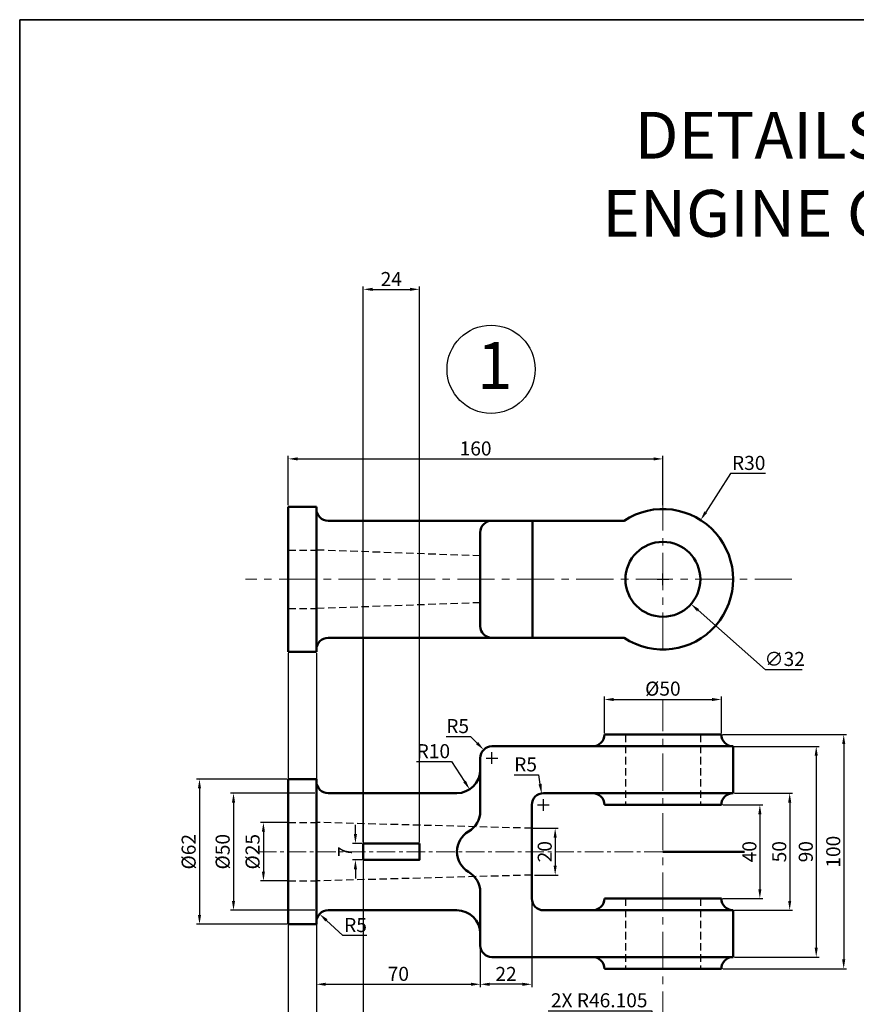
# Model space of a CAD drawing. Units: millimetres. Extents: x 208 to 901, y -26 to 704.
# Tile 2 of 3: x 208 to 566, y 283 to 704. Entities that reach past the tile are written whole.
import ezdxf

# ---------------------------------------------------------------- set-up
doc = ezdxf.new("R2010")
doc.units = ezdxf.units.MM
doc.header["$LTSCALE"] = 0.5
doc.linetypes.add('CENTER', pattern=[50.8, 31.75, -6.35, 6.35, -6.35])
doc.linetypes.add('DASHED', pattern=[19.05, 12.7, -6.35])
for name, color, linetype, lineweight in [('M-CNTR', 1, 'CENTER', 18), ('M-DIMS', 2, 'Continuous', 25), ('M-HIDN', 6, 'DASHED', 25), ('M-OUTL', 7, 'Continuous', 50), ('M-TEXT', 3, 'Continuous', 25), ('M-TTLB', 7, 'Continuous', 35)]:
    doc.layers.add(name, color=color, linetype=linetype, lineweight=lineweight)
doc.styles.get("Standard").update_dxf_attribs({"font": 'arial.ttf'})
doc.dimstyles.new('ISO-25', dxfattribs={"dimtxt": 6, "dimasz": 4, "dimexe": 1.25, "dimexo": 0.625, "dimtad": 1, "dimtoh": 1, "dimdec": 0, "dimtxsty": 'Standard', "dimcen": 2.5, "dimadec": 0, "dimazin": 0, "dimtfac": 1, "dimtdec": 0, "dimtofl": 0, "dimtmove": 0, "dimatfit": 3, "dimfxl": 1, "dimarcsym": 0})

# ---------------------------------------------------------------- blocks, each defined once
blk = doc.blocks.new('*D1')
at = {"layer": 'Defpoints', "color": 0, "ltscale": 0.5, "transparency": 16777216}
for p in [(483.01, 516.18), (323.01, 495.77), (483.01, 495.77)]:
    blk.add_point(p, dxfattribs=at)
at = {"layer": 'M-DIMS', "color": 0, "lineweight": -2, "ltscale": 0.5, "transparency": 16777216}
for p, q in [((323.01, 496.4), (323.01, 517.43)), ((483.01, 496.4), (483.01, 517.43)), ((327.01, 516.18), (479.01, 516.18))]:
    blk.add_line(p, q, dxfattribs=at)
at = {"layer": 'M-DIMS', "color": 0, "ltscale": 0.5, "transparency": 16777216}
for points in [[(327.01, 516.84), (327.01, 515.51), (323.01, 516.18)], [(479.01, 516.84), (479.01, 515.51), (483.01, 516.18)]]:
    blk.add_solid(points, dxfattribs=at)
at = {"layer": 'M-DIMS', "color": 0, "ltscale": 0.5, "transparency": 16777216, "insert": (403.01, 519.86), "char_height": 6, "attachment_point": 5}
blk.add_mtext('160', dxfattribs=at)
blk = doc.blocks.new('*D2')
at = {"layer": 'Defpoints', "color": 0, "ltscale": 0.5, "transparency": 16777216}
for p in [(471.01, 475.35), (495.02, 454.19)]:
    blk.add_point(p, dxfattribs=at)
at = {"layer": 'M-DIMS', "color": 0, "lineweight": -2, "ltscale": 0.5, "transparency": 16777216}
for p, q in [((483.01, 462.27), (483.01, 467.27)), ((480.51, 464.77), (485.51, 464.77)), ((526.89, 426.11), (498.02, 451.55)), ((542.57, 426.11), (526.89, 426.11))]:
    blk.add_line(p, q, dxfattribs=at)
at = {"layer": 'M-DIMS', "color": 0, "ltscale": 0.5, "transparency": 16777216}
blk.add_solid([(498.46, 452.05), (497.58, 451.05), (495.02, 454.19)], dxfattribs=at)
at = {"layer": 'M-DIMS', "color": 0, "ltscale": 0.5, "transparency": 16777216, "insert": (535.04, 429.96), "char_height": 6, "attachment_point": 5}
blk.add_mtext('∅32', dxfattribs=at)
blk = doc.blocks.new('*D3')
at = {"layer": 'Defpoints', "color": 0, "ltscale": 0.5, "transparency": 16777216}
for p in [(499.16, 490.06), (483.01, 464.77)]:
    blk.add_point(p, dxfattribs=at)
at = {"layer": 'M-DIMS', "color": 0, "lineweight": -2, "ltscale": 0.5, "transparency": 16777216}
for p, q in [((511.88, 509.99), (501.31, 493.43)), ((526.82, 509.99), (511.88, 509.99)), ((483.01, 462.27), (483.01, 467.27)), ((480.51, 464.77), (485.51, 464.77))]:
    blk.add_line(p, q, dxfattribs=at)
at = {"layer": 'M-DIMS', "color": 0, "ltscale": 0.5, "transparency": 16777216}
blk.add_solid([(500.75, 493.79), (501.87, 493.07), (499.16, 490.06)], dxfattribs=at)
at = {"layer": 'M-DIMS', "color": 0, "ltscale": 0.5, "transparency": 16777216, "insert": (519.67, 513.68), "char_height": 6, "attachment_point": 5}
blk.add_mtext('R30', dxfattribs=at)
blk = doc.blocks.new('*D4')
at = {"layer": 'Defpoints', "color": 0, "ltscale": 0.5, "transparency": 16777216}
for p in [(355.01, 351.93), (351.68, 344.93), (355.01, 344.93)]:
    blk.add_point(p, dxfattribs=at)
at = {"layer": 'M-DIMS', "color": 0, "lineweight": -2, "ltscale": 0.5, "transparency": 16777216}
for p, q in [((351.68, 355.93), (351.68, 359.93)), ((354.39, 351.93), (350.43, 351.93)), ((354.39, 344.93), (350.43, 344.93)), ((351.68, 340.93), (351.68, 336.93))]:
    blk.add_line(p, q, dxfattribs=at)
at = {"layer": 'M-DIMS', "color": 0, "ltscale": 0.5, "transparency": 16777216}
for points in [[(351.01, 355.93), (352.34, 355.93), (351.68, 351.93)], [(351.01, 340.93), (352.34, 340.93), (351.68, 344.93)]]:
    blk.add_solid(points, dxfattribs=at)
at = {"layer": 'M-DIMS', "color": 0, "ltscale": 0.5, "transparency": 16777216, "insert": (348.05, 348.43), "char_height": 6, "attachment_point": 5, "rotation": 90}
blk.add_mtext('7', dxfattribs=at)
blk = doc.blocks.new('*D5')
at = {"layer": 'Defpoints', "color": 0, "ltscale": 0.5, "transparency": 16777216}
for p in [(323.01, 360.93), (312.38, 335.93), (323.01, 335.93)]:
    blk.add_point(p, dxfattribs=at)
at = {"layer": 'M-DIMS', "color": 0, "lineweight": -2, "ltscale": 0.5, "transparency": 16777216}
for p, q in [((322.39, 360.93), (311.13, 360.93)), ((312.38, 356.93), (312.38, 339.93)), ((322.39, 335.93), (311.13, 335.93))]:
    blk.add_line(p, q, dxfattribs=at)
at = {"layer": 'M-DIMS', "color": 0, "ltscale": 0.5, "transparency": 16777216}
for points in [[(311.71, 356.93), (313.04, 356.93), (312.38, 360.93)], [(311.71, 339.93), (313.04, 339.93), (312.38, 335.93)]]:
    blk.add_solid(points, dxfattribs=at)
at = {"layer": 'M-DIMS', "color": 0, "ltscale": 0.5, "transparency": 16777216, "insert": (308.52, 348.43), "char_height": 6, "attachment_point": 5, "rotation": 90}
blk.add_mtext('%%C25', dxfattribs=at)
blk = doc.blocks.new('*D6')
at = {"layer": 'Defpoints', "color": 0, "ltscale": 0.5, "transparency": 16777216}
for p in [(335.01, 373.43), (299.6, 323.43), (335.01, 323.43)]:
    blk.add_point(p, dxfattribs=at)
at = {"layer": 'M-DIMS', "color": 0, "lineweight": -2, "ltscale": 0.5, "transparency": 16777216}
for p, q in [((334.39, 373.43), (298.35, 373.43)), ((299.6, 369.43), (299.6, 327.43)), ((334.39, 323.43), (298.35, 323.43))]:
    blk.add_line(p, q, dxfattribs=at)
at = {"layer": 'M-DIMS', "color": 0, "ltscale": 0.5, "transparency": 16777216}
for points in [[(298.93, 369.43), (300.27, 369.43), (299.6, 373.43)], [(298.93, 327.43), (300.27, 327.43), (299.6, 323.43)]]:
    blk.add_solid(points, dxfattribs=at)
at = {"layer": 'M-DIMS', "color": 0, "ltscale": 0.5, "transparency": 16777216, "insert": (295.74, 348.43), "char_height": 6, "attachment_point": 5, "rotation": 90}
blk.add_mtext('%%C50', dxfattribs=at)
blk = doc.blocks.new('*D7')
at = {"layer": 'Defpoints', "color": 0, "ltscale": 0.5, "transparency": 16777216}
for p in [(323.01, 379.43), (285.06, 317.43), (323.01, 317.43)]:
    blk.add_point(p, dxfattribs=at)
at = {"layer": 'M-DIMS', "color": 0, "lineweight": -2, "ltscale": 0.5, "transparency": 16777216}
for p, q in [((322.39, 379.43), (283.81, 379.43)), ((285.06, 375.43), (285.06, 321.43)), ((322.39, 317.43), (283.81, 317.43))]:
    blk.add_line(p, q, dxfattribs=at)
at = {"layer": 'M-DIMS', "color": 0, "ltscale": 0.5, "transparency": 16777216}
for points in [[(284.4, 375.43), (285.73, 375.43), (285.06, 379.43)], [(284.4, 321.43), (285.73, 321.43), (285.06, 317.43)]]:
    blk.add_solid(points, dxfattribs=at)
at = {"layer": 'M-DIMS', "color": 0, "ltscale": 0.5, "transparency": 16777216, "insert": (281.21, 348.43), "char_height": 6, "attachment_point": 5, "rotation": 90}
blk.add_mtext('%%C62', dxfattribs=at)
blk = doc.blocks.new('*D8')
at = {"layer": 'Defpoints', "color": 0, "ltscale": 0.5, "transparency": 16777216}
for p in [(335.01, 317.43), (405.01, 313.43), (405.01, 291.81)]:
    blk.add_point(p, dxfattribs=at)
at = {"layer": 'M-DIMS', "color": 0, "lineweight": -2, "ltscale": 0.5, "transparency": 16777216}
for p, q in [((335.01, 316.81), (335.01, 290.56)), ((405.01, 312.81), (405.01, 290.56)), ((339.01, 291.81), (401.01, 291.81))]:
    blk.add_line(p, q, dxfattribs=at)
at = {"layer": 'M-DIMS', "color": 0, "ltscale": 0.5, "transparency": 16777216}
for points in [[(339.01, 292.48), (339.01, 291.14), (335.01, 291.81)], [(401.01, 292.48), (401.01, 291.14), (405.01, 291.81)]]:
    blk.add_solid(points, dxfattribs=at)
at = {"layer": 'M-DIMS', "color": 0, "ltscale": 0.5, "transparency": 16777216, "insert": (370.01, 295.5), "char_height": 6, "attachment_point": 5}
blk.add_mtext('70', dxfattribs=at)
blk = doc.blocks.new('*D9')
at = {"layer": 'Defpoints', "color": 0, "ltscale": 0.5, "transparency": 16777216}
for p in [(427.01, 333.71), (405.01, 301.68), (405.01, 291.81)]:
    blk.add_point(p, dxfattribs=at)
at = {"layer": 'M-DIMS', "color": 0, "lineweight": -2, "ltscale": 0.5, "transparency": 16777216}
for p, q in [((427.01, 333.08), (427.01, 290.56)), ((405.01, 301.06), (405.01, 290.56)), ((423.01, 291.81), (409.01, 291.81))]:
    blk.add_line(p, q, dxfattribs=at)
at = {"layer": 'M-DIMS', "color": 0, "ltscale": 0.5, "transparency": 16777216}
for points in [[(409.01, 292.48), (409.01, 291.14), (405.01, 291.81)], [(423.01, 292.48), (423.01, 291.14), (427.01, 291.81)]]:
    blk.add_solid(points, dxfattribs=at)
at = {"layer": 'M-DIMS', "color": 0, "ltscale": 0.5, "transparency": 16777216, "insert": (416.01, 295.45), "char_height": 6, "attachment_point": 5}
blk.add_mtext('22', dxfattribs=at)
blk = doc.blocks.new('*D10')
at = {"layer": 'Defpoints', "color": 0, "ltscale": 0.5, "transparency": 16777216}
for p in [(427.01, 358.43), (427.56, 338.45), (437.01, 338.45)]:
    blk.add_point(p, dxfattribs=at)
at = {"layer": 'M-DIMS', "color": 0, "lineweight": -2, "ltscale": 0.5, "transparency": 16777216}
for p, q in [((427.64, 358.43), (438.26, 358.43)), ((437.01, 354.43), (437.01, 342.45)), ((428.18, 338.45), (438.26, 338.45))]:
    blk.add_line(p, q, dxfattribs=at)
at = {"layer": 'M-DIMS', "color": 0, "ltscale": 0.5, "transparency": 16777216}
for points in [[(436.34, 354.43), (437.67, 354.43), (437.01, 358.43)], [(436.34, 342.45), (437.67, 342.45), (437.01, 338.45)]]:
    blk.add_solid(points, dxfattribs=at)
at = {"layer": 'M-DIMS', "color": 0, "ltscale": 0.5, "transparency": 16777216, "insert": (433.32, 348.44), "char_height": 6, "attachment_point": 5, "rotation": 90}
blk.add_mtext('20', dxfattribs=at)
blk = doc.blocks.new('*D11')
at = {"layer": 'Defpoints', "color": 0, "ltscale": 0.5, "transparency": 16777216}
for p in [(508.01, 413.43), (458.01, 398.43), (508.01, 398.43)]:
    blk.add_point(p, dxfattribs=at)
at = {"layer": 'M-DIMS', "color": 0, "lineweight": -2, "ltscale": 0.5, "transparency": 16777216}
for p, q in [((458.01, 399.06), (458.01, 414.68)), ((462.01, 413.43), (504.01, 413.43)), ((508.01, 399.06), (508.01, 414.68))]:
    blk.add_line(p, q, dxfattribs=at)
at = {"layer": 'M-DIMS', "color": 0, "ltscale": 0.5, "transparency": 16777216}
for points in [[(462.01, 414.1), (462.01, 412.77), (458.01, 413.43)], [(504.01, 414.1), (504.01, 412.77), (508.01, 413.43)]]:
    blk.add_solid(points, dxfattribs=at)
at = {"layer": 'M-DIMS', "color": 0, "ltscale": 0.5, "transparency": 16777216, "insert": (483.01, 417.29), "char_height": 6, "attachment_point": 5}
blk.add_mtext('%%C50', dxfattribs=at)
blk = doc.blocks.new('*D12')
at = {"layer": 'Defpoints', "color": 0, "ltscale": 0.5, "transparency": 16777216}
for p in [(508.01, 368.43), (508.01, 328.43), (524.44, 328.43)]:
    blk.add_point(p, dxfattribs=at)
at = {"layer": 'M-DIMS', "color": 0, "lineweight": -2, "ltscale": 0.5, "transparency": 16777216}
for p, q in [((508.64, 368.43), (525.69, 368.43)), ((524.44, 364.43), (524.44, 332.43)), ((508.64, 328.43), (525.69, 328.43))]:
    blk.add_line(p, q, dxfattribs=at)
at = {"layer": 'M-DIMS', "color": 0, "ltscale": 0.5, "transparency": 16777216}
for points in [[(523.77, 364.43), (525.1, 364.43), (524.44, 368.43)], [(523.77, 332.43), (525.1, 332.43), (524.44, 328.43)]]:
    blk.add_solid(points, dxfattribs=at)
at = {"layer": 'M-DIMS', "color": 0, "ltscale": 0.5, "transparency": 16777216, "insert": (520.75, 348.43), "char_height": 6, "attachment_point": 5, "rotation": 90}
blk.add_mtext('40', dxfattribs=at)
blk = doc.blocks.new('*D13')
at = {"layer": 'Defpoints', "color": 0, "ltscale": 0.5, "transparency": 16777216}
for p in [(513.01, 373.43), (513.01, 323.43), (537.19, 323.43)]:
    blk.add_point(p, dxfattribs=at)
at = {"layer": 'M-DIMS', "color": 0, "lineweight": -2, "ltscale": 0.5, "transparency": 16777216}
for p, q in [((513.64, 373.43), (538.44, 373.43)), ((537.19, 369.43), (537.19, 327.43)), ((513.64, 323.43), (538.44, 323.43))]:
    blk.add_line(p, q, dxfattribs=at)
at = {"layer": 'M-DIMS', "color": 0, "ltscale": 0.5, "transparency": 16777216}
for points in [[(536.52, 369.43), (537.85, 369.43), (537.19, 373.43)], [(536.52, 327.43), (537.85, 327.43), (537.19, 323.43)]]:
    blk.add_solid(points, dxfattribs=at)
at = {"layer": 'M-DIMS', "color": 0, "ltscale": 0.5, "transparency": 16777216, "insert": (533.5, 348.43), "char_height": 6, "attachment_point": 5, "rotation": 90}
blk.add_mtext('50', dxfattribs=at)
blk = doc.blocks.new('*D14')
at = {"layer": 'Defpoints', "color": 0, "ltscale": 0.5, "transparency": 16777216}
for p in [(513.01, 393.43), (513.01, 303.43), (548.52, 303.43)]:
    blk.add_point(p, dxfattribs=at)
at = {"layer": 'M-DIMS', "color": 0, "lineweight": -2, "ltscale": 0.5, "transparency": 16777216}
for p, q in [((513.64, 393.43), (549.77, 393.43)), ((548.52, 389.43), (548.52, 307.43)), ((513.64, 303.43), (549.77, 303.43))]:
    blk.add_line(p, q, dxfattribs=at)
at = {"layer": 'M-DIMS', "color": 0, "ltscale": 0.5, "transparency": 16777216}
for points in [[(547.85, 389.43), (549.19, 389.43), (548.52, 393.43)], [(547.85, 307.43), (549.19, 307.43), (548.52, 303.43)]]:
    blk.add_solid(points, dxfattribs=at)
at = {"layer": 'M-DIMS', "color": 0, "ltscale": 0.5, "transparency": 16777216, "insert": (544.83, 348.43), "char_height": 6, "attachment_point": 5, "rotation": 90}
blk.add_mtext('90', dxfattribs=at)
blk = doc.blocks.new('*D15')
at = {"layer": 'Defpoints', "color": 0, "ltscale": 0.5, "transparency": 16777216}
for p in [(508.01, 398.43), (508.01, 298.43), (560.26, 298.43)]:
    blk.add_point(p, dxfattribs=at)
at = {"layer": 'M-DIMS', "color": 0, "lineweight": -2, "ltscale": 0.5, "transparency": 16777216}
for p, q in [((508.64, 398.43), (561.51, 398.43)), ((560.26, 394.43), (560.26, 302.43)), ((508.64, 298.43), (561.51, 298.43))]:
    blk.add_line(p, q, dxfattribs=at)
at = {"layer": 'M-DIMS', "color": 0, "ltscale": 0.5, "transparency": 16777216}
for points in [[(559.59, 394.43), (560.92, 394.43), (560.26, 398.43)], [(559.59, 302.43), (560.92, 302.43), (560.26, 298.43)]]:
    blk.add_solid(points, dxfattribs=at)
at = {"layer": 'M-DIMS', "color": 0, "ltscale": 0.5, "transparency": 16777216, "insert": (556.57, 348.43), "char_height": 6, "attachment_point": 5, "rotation": 90}
blk.add_mtext('100', dxfattribs=at)
blk = doc.blocks.new('*D16')
at = {"layer": 'Defpoints', "color": 0, "ltscale": 0.5, "transparency": 16777216}
for p in [(406.48, 391.97), (410.01, 388.43)]:
    blk.add_point(p, dxfattribs=at)
at = {"layer": 'M-DIMS', "color": 0, "lineweight": -2, "ltscale": 0.5, "transparency": 16777216}
for p, q in [((390.48, 397.63), (400.82, 397.63)), ((400.82, 397.63), (403.65, 394.8)), ((407.51, 388.43), (412.51, 388.43)), ((410.01, 385.93), (410.01, 390.93))]:
    blk.add_line(p, q, dxfattribs=at)
at = {"layer": 'M-DIMS', "color": 0, "ltscale": 0.5, "transparency": 16777216}
blk.add_solid([(404.12, 395.27), (403.18, 394.33), (406.48, 391.97)], dxfattribs=at)
at = {"layer": 'M-DIMS', "color": 0, "ltscale": 0.5, "transparency": 16777216, "insert": (395.34, 401.3), "char_height": 6, "attachment_point": 5}
blk.add_mtext('R5', dxfattribs=at)
blk = doc.blocks.new('*D17')
at = {"layer": 'Defpoints', "color": 0, "ltscale": 0.5, "transparency": 16777216}
for p in [(395.01, 383.43), (400.49, 375.07)]:
    blk.add_point(p, dxfattribs=at)
at = {"layer": 'M-DIMS', "color": 0, "lineweight": -2, "ltscale": 0.5, "transparency": 16777216}
for p, q in [((377.81, 386.89), (392.75, 386.89)), ((392.75, 386.89), (398.3, 378.41))]:
    blk.add_line(p, q, dxfattribs=at)
at = {"layer": 'M-DIMS', "color": 0, "ltscale": 0.5, "transparency": 16777216}
blk.add_solid([(398.86, 378.78), (397.74, 378.05), (400.49, 375.07)], dxfattribs=at)
at = {"layer": 'M-DIMS', "color": 0, "ltscale": 0.5, "transparency": 16777216, "insert": (384.97, 390.58), "char_height": 6, "attachment_point": 5}
blk.add_mtext('R10', dxfattribs=at)
blk = doc.blocks.new('*D18')
at = {"layer": 'Defpoints', "color": 0, "ltscale": 0.5, "transparency": 16777216}
for p in [(336.35, 321.83), (340.01, 318.43)]:
    blk.add_point(p, dxfattribs=at)
at = {"layer": 'M-DIMS', "color": 0, "lineweight": -2, "ltscale": 0.5, "transparency": 16777216}
for p, q in [((346.23, 312.66), (339.28, 319.11)), ((356.58, 312.66), (346.23, 312.66))]:
    blk.add_line(p, q, dxfattribs=at)
at = {"layer": 'M-DIMS', "color": 0, "ltscale": 0.5, "transparency": 16777216}
blk.add_solid([(339.73, 319.6), (338.83, 318.62), (336.35, 321.83)], dxfattribs=at)
at = {"layer": 'M-DIMS', "color": 0, "ltscale": 0.5, "transparency": 16777216, "insert": (351.72, 316.34), "char_height": 6, "attachment_point": 5}
blk.add_mtext('R5', dxfattribs=at)
blk = doc.blocks.new('*D19')
at = {"layer": 'Defpoints', "color": 0, "ltscale": 0.5, "transparency": 16777216}
for p in [(431.18, 373.36), (432.01, 368.43)]:
    blk.add_point(p, dxfattribs=at)
at = {"layer": 'M-DIMS', "color": 0, "lineweight": -2, "ltscale": 0.5, "transparency": 16777216}
for p, q in [((419.5, 381.25), (429.85, 381.25)), ((429.85, 381.25), (430.51, 377.31)), ((432.01, 365.93), (432.01, 370.93)), ((429.51, 368.43), (434.51, 368.43))]:
    blk.add_line(p, q, dxfattribs=at)
at = {"layer": 'M-DIMS', "color": 0, "ltscale": 0.5, "transparency": 16777216}
blk.add_solid([(431.17, 377.42), (429.86, 377.2), (431.18, 373.36)], dxfattribs=at)
at = {"layer": 'M-DIMS', "color": 0, "ltscale": 0.5, "transparency": 16777216, "insert": (424.36, 384.93), "char_height": 6, "attachment_point": 5}
blk.add_mtext('R5', dxfattribs=at)
blk = doc.blocks.new('*D50')
at = {"layer": 'Defpoints', "color": 0, "ltscale": 0.5, "transparency": 16777216}
for p in [(323.01, 433.77), (335.01, 433.77), (335.01, 257.57)]:
    blk.add_point(p, dxfattribs=at)
at = {"layer": 'M-DIMS', "color": 0, "lineweight": -2, "ltscale": 0.5, "transparency": 16777216}
for p, q in [((323.01, 433.15), (323.01, 256.32)), ((335.01, 433.15), (335.01, 256.32)), ((327.01, 257.57), (331.01, 257.57))]:
    blk.add_line(p, q, dxfattribs=at)
at = {"layer": 'M-DIMS', "color": 0, "ltscale": 0.5, "transparency": 16777216}
for points in [[(327.01, 258.24), (327.01, 256.91), (323.01, 257.57)], [(331.01, 258.24), (331.01, 256.91), (335.01, 257.57)]]:
    blk.add_solid(points, dxfattribs=at)
at = {"layer": 'M-DIMS', "color": 0, "ltscale": 0.5, "transparency": 16777216, "insert": (329.01, 261.21), "char_height": 6, "attachment_point": 5}
blk.add_mtext('12', dxfattribs=at)
blk = doc.blocks.new('*D51')
at = {"layer": 'Defpoints', "color": 0, "ltscale": 0.5, "transparency": 16777216}
for p in [(379.01, 588.59), (355.01, 351.93), (379.01, 351.93)]:
    blk.add_point(p, dxfattribs=at)
at = {"layer": 'M-DIMS', "color": 0, "lineweight": -2, "ltscale": 0.5, "transparency": 16777216}
for p, q in [((355.01, 352.56), (355.01, 589.84)), ((379.01, 352.56), (379.01, 589.84)), ((359.01, 588.59), (375.01, 588.59))]:
    blk.add_line(p, q, dxfattribs=at)
at = {"layer": 'M-DIMS', "color": 0, "ltscale": 0.5, "transparency": 16777216}
for points in [[(359.01, 589.25), (359.01, 587.92), (355.01, 588.59)], [(375.01, 589.25), (375.01, 587.92), (379.01, 588.59)]]:
    blk.add_solid(points, dxfattribs=at)
at = {"layer": 'M-DIMS', "color": 0, "ltscale": 0.5, "transparency": 16777216, "insert": (367.01, 592.22), "char_height": 6, "attachment_point": 5}
blk.add_mtext('24', dxfattribs=at)
blk = doc.blocks.new('*D52')
at = {"layer": 'Defpoints', "color": 0, "ltscale": 0.5, "transparency": 16777216}
for p in [(355.01, 439.77), (335.01, 433.77), (355.01, 257.57)]:
    blk.add_point(p, dxfattribs=at)
at = {"layer": 'M-DIMS', "color": 0, "lineweight": -2, "ltscale": 0.5, "transparency": 16777216}
for p, q in [((355.01, 439.15), (355.01, 256.32)), ((335.01, 433.15), (335.01, 256.32)), ((339.01, 257.57), (351.01, 257.57))]:
    blk.add_line(p, q, dxfattribs=at)
at = {"layer": 'M-DIMS', "color": 0, "ltscale": 0.5, "transparency": 16777216}
for points in [[(339.01, 258.24), (339.01, 256.91), (335.01, 257.57)], [(351.01, 258.24), (351.01, 256.91), (355.01, 257.57)]]:
    blk.add_solid(points, dxfattribs=at)
at = {"layer": 'M-DIMS', "color": 0, "ltscale": 0.5, "transparency": 16777216, "insert": (345.01, 261.26), "char_height": 6, "attachment_point": 5}
blk.add_mtext('20', dxfattribs=at)
blk = doc.blocks.new('*D54')
at = {"layer": 'Defpoints', "color": 0, "ltscale": 0.5, "transparency": 16777216}
for p in [(478.3, 252.85), (478.31, 206.74)]:
    blk.add_point(p, dxfattribs=at)
at = {"layer": 'M-DIMS', "color": 0, "lineweight": -2, "ltscale": 0.5, "transparency": 16777216}
for p, q in [((433.98, 280.51), (478.29, 280.51)), ((478.29, 280.51), (478.3, 256.85)), ((475.81, 206.74), (480.81, 206.74)), ((478.31, 204.24), (478.31, 209.24))]:
    blk.add_line(p, q, dxfattribs=at)
at = {"layer": 'M-DIMS', "color": 0, "ltscale": 0.5, "transparency": 16777216}
blk.add_solid([(478.97, 256.85), (477.63, 256.85), (478.3, 252.85)], dxfattribs=at)
at = {"layer": 'M-DIMS', "color": 0, "ltscale": 0.5, "transparency": 16777216, "insert": (455.82, 284.2), "char_height": 6, "attachment_point": 5}
blk.add_mtext('2X R46.105', dxfattribs=at)

msp = doc.modelspace()

# ---------------------------------------------------------------- linework, layer by layer
at = {"layer": 'M-CNTR'}
for p, q in [((483.0137, 434.7711), (483.0137, 513.015)), ((538.1121, 464.7711), (304.7661, 464.7711)), ((483.0137, 272.8724), (483.0137, 413.4329))]:
    msp.add_line(p, q, dxfattribs=at)
at = {"layer": 'M-CNTR', "ltscale": 0.5}
msp.add_line((483.0137, 348.4335), (310.7143, 348.4335), dxfattribs=at)
at = {"layer": 'M-HIDN', "ltscale": 0.5}
for p, q in [((355.0137, 476.5568), (355.0137, 489.7711)), ((379.0137, 475.6997), (379.0137, 489.7711)), ((323.0137, 477.2711), (335.0137, 477.2711)), ((405.0137, 474.7711), (335.0137, 477.2711)), ((405.0137, 454.7711), (335.0137, 452.2711)), ((323.0137, 452.2711), (335.0137, 452.2711)), ((355.0137, 439.7711), (355.0137, 452.9854)), ((379.0137, 439.7711), (379.0137, 453.8426)), ((467.0137, 398.4335), (467.0137, 368.4335)), ((499.0137, 398.4335), (499.0137, 368.4335)), ((323.0137, 360.9335), (335.0137, 360.9335)), ((427.0137, 358.4335), (335.0137, 360.9335)), ((427.0137, 338.4335), (335.0137, 335.9335)), ((323.0137, 335.9335), (335.0137, 335.9335)), ((467.0137, 328.4335), (467.0137, 298.4335)), ((499.0137, 328.4335), (499.0137, 298.4335))]:
    msp.add_line(p, q, dxfattribs=at)
at = {"layer": 'M-OUTL'}
for p, q in [((323.0137, 464.7711), (323.0137, 495.7711)), ((323.0137, 495.7711), (335.0137, 495.7711)), ((335.0137, 495.7711), (335.0137, 494.7711)), ((340.0137, 489.7711), (466.4306, 489.7711)), ((323.0137, 433.7711), (323.0137, 464.7711)), ((340.0137, 439.7711), (466.4306, 439.7711)), ((335.0137, 433.7711), (323.0137, 433.7711)), ((335.0137, 434.7711), (335.0137, 433.7711))]:
    msp.add_line(p, q, dxfattribs=at)
at = {"layer": 'M-OUTL', "ltscale": 0.5}
for p, q in [((335.0137, 433.7711), (335.0137, 495.7711)), ((427.2783, 439.7711), (427.2783, 489.7711)), ((405.0137, 444.7711), (405.0137, 484.7711)), ((508.0137, 398.4335), (458.0137, 398.4335)), ((458.0137, 398.4335), (458.0137, 398.4335)), ((508.0137, 398.4335), (508.0137, 398.4335)), ((410.0137, 393.4335), (513.0137, 393.4335)), ((513.0137, 393.4335), (513.0137, 393.4335)), ((513.0137, 393.4335), (513.0137, 373.4335)), ((405.0137, 388.4335), (405.0137, 383.4335)), ((405.0137, 385.9335), (405.0137, 388.4335)), ((405.0137, 383.4335), (405.0137, 365.754)), ((432.0137, 373.4335), (513.0137, 373.4335)), ((453.0137, 373.4335), (453.0137, 373.4335)), ((513.0137, 373.4335), (513.0137, 373.4335)), ((427.0137, 368.4335), (427.0137, 328.4335)), ((458.0137, 368.4335), (508.0137, 368.4335)), ((458.0137, 368.4335), (458.0137, 368.4335)), ((508.0137, 368.4335), (508.0137, 368.4335)), ((483.0137, 348.4335), (517.8486, 348.4335)), ((405.0137, 308.4335), (405.0137, 331.113)), ((458.0137, 328.4335), (458.0137, 328.4335)), ((458.0137, 328.4335), (508.0137, 328.4335)), ((508.0137, 328.4335), (508.0137, 328.4335)), ((432.0137, 323.4335), (513.0137, 323.4335)), ((453.0137, 323.4335), (453.0137, 323.4335)), ((513.0137, 323.4335), (513.0137, 323.4335)), ((513.0137, 303.4335), (513.0137, 323.4335)), ((335.0137, 317.4335), (323.0137, 317.4335)), ((405.0137, 318.4335), (405.0137, 308.4335)), ((405.0137, 313.4335), (405.0137, 308.4335)), ((410.0137, 303.4335), (513.0137, 303.4335)), ((513.0137, 303.4335), (513.0137, 303.4335)), ((508.0137, 298.4335), (458.0137, 298.4335)), ((458.0137, 298.4335), (458.0137, 298.4335)), ((508.0137, 298.4335), (508.0137, 298.4335))]:
    msp.add_line(p, q, dxfattribs=at)
for points in [[(323.0137, 317.4335), (323.0137, 348.4335), (323.0137, 379.4335), (335.0137, 379.4335), (335.0137, 378.4335, 0.41421356), (340.0137, 373.4335), (395.0137, 373.4335)], [(395.0137, 323.4335), (340.0137, 323.4335, 0.41421356), (335.0137, 318.4335), (335.0137, 317.4335)]]:
    msp.add_lwpolyline(points, format="xyb", dxfattribs=at)
msp.add_lwpolyline([(335.0137, 378.4335), (335.0137, 318.4335)], dxfattribs=at)
msp.add_lwpolyline([(379.0137, 351.9335), (379.0137, 344.9335), (355.0137, 344.9335), (355.0137, 348.4335), (355.0137, 351.9335)], close=True, dxfattribs=at)
at = {"layer": 'M-OUTL'}
msp.add_circle((483.0137, 464.7711), 16, dxfattribs=at)
for centre, radius, start, end in [((340.0137, 494.7711), 5, 180, 270), ((483.0137, 464.7711), 30, 236.44269, 123.55731), ((410.0137, 484.7711), 5, 90, 180), ((410.0137, 444.7711), 5, 180, 270), ((340.0137, 434.7711), 5, 90, 180)]:
    msp.add_arc(centre, radius, start, end, dxfattribs=at)
at = {"layer": 'M-OUTL', "ltscale": 0.5}
for centre, radius, start, end in [((453.0137, 398.4335), 5, 270, 0), ((513.0137, 398.4335), 5, 180, 270), ((410.0137, 388.4335), 5, 90, 180), ((395.0137, 383.4335), 10, 270, 0), ((432.0137, 368.4335), 5, 90, 180), ((453.0137, 368.4335), 5, 0, 90), ((513.0137, 368.4335), 5, 90, 180), ((395.0137, 365.754), 10, 300, 0), ((405.0137, 348.4335), 10, 120, 240), ((395.0137, 331.113), 10, 0, 60), ((432.0137, 328.4335), 5, 180, 270), ((453.0137, 328.4335), 5, 270, 0), ((513.0137, 328.4335), 5, 180, 270), ((395.0137, 313.4335), 10, 0, 90), ((410.0137, 308.4335), 5, 180, 270), ((453.0137, 298.4335), 5, 0, 90), ((513.0137, 298.4335), 5, 90, 180)]:
    msp.add_arc(centre, radius, start, end, dxfattribs=at)
at = {"layer": 'M-TEXT', "ltscale": 0.5}
msp.add_circle((409.629, 554.4598), 18.8257, dxfattribs=at)
at = {"layer": 'M-TTLB', "ltscale": 0.5}
msp.add_lwpolyline([(208.2585, 703.7432), (900.8689, 703.7432), (900.8689, -25.914), (208.2585, -25.914)], close=True, dxfattribs=at)

# ---------------------------------------------------------------- texts
at = {"layer": 'M-TEXT', "ltscale": 0.5, "char_height": 20, "attachment_point": 1}
for s, width, insert in [('\\pxqc;DETAILS OF STEAM ENGINE CROSS HEAD', 309.964733, (436.8417, 664.3913)), ('1', 20, (403.5732, 566.0959))]:
    msp.add_mtext_dynamic_manual_height_columns(s, width=width, gutter_width=12.5, heights=[0], dxfattribs=dict(at, insert=insert))

# ---------------------------------------------------------------- dimensions: what is measured, and where the dimension line sits
at = {"layer": 'M-DIMS', "ltscale": 0.5}
for base, p1, p2, override, picture, middle in [((379.0137, 588.5855), (355.0137, 351.9335), (379.0137, 351.9335), {"dimdec": 0, "dimlfac": 1, "dimrnd": 0, "dimzin": 0, "dimdsep": 46, "dimlunit": 2}, '*D51', (367.0137, 592.2228)), ((483.0137, 516.1755), (323.0137, 495.7711), (483.0137, 495.7711), {"dimclrd": 0, "dimclre": 0, "dimclrt": 0}, '*D1', (403.0137, 519.864)), ((355.0137, 257.5724), (335.0137, 433.7711), (355.0137, 439.7711), {"dimdec": 0, "dimlfac": 1, "dimrnd": 0, "dimzin": 0, "dimdsep": 46, "dimlunit": 2}, '*D52', (345.0137, 261.2608)), ((335.0137, 257.5724), (323.0137, 433.7711), (335.0137, 433.7711), {"dimdec": 0, "dimlfac": 1, "dimrnd": 0, "dimzin": 0, "dimdsep": 46, "dimlunit": 2}, '*D50', (329.0137, 261.2096)), ((405.0137, 291.809), (427.0137, 333.7092), (405.0137, 301.6838), {"dimclrd": 0, "dimclre": 0, "dimclrt": 0}, '*D9', (416.0137, 295.4463)), ((405.0137, 291.809), (335.0137, 317.4335), (405.0137, 313.4335), {"dimclrd": 0, "dimclre": 0, "dimclrt": 0}, '*D8', (370.0137, 295.4975))]:
    dim = msp.add_linear_dim(base=base, p1=p1, p2=p2, dimstyle='ISO-25', override=override, dxfattribs=at)
    dim.commit()
    dim.dimension.update_dxf_attribs({"geometry": picture, "text_midpoint": middle})
for center, mpoint, picture, middle in [((483.0137, 464.7711), (499.1579, 490.0568), '*D3', (519.6667, 509.9881)), ((395.0137, 383.4335), (400.4897, 375.0661), '*D17', (384.9706, 386.8866)), ((340.0137, 318.4335), (336.3485, 321.8344), '*D18', (351.719, 312.6621))]:
    dim = msp.add_radius_dim(center=center, mpoint=mpoint, dimstyle='ISO-25', override={"dimclrd": 0, "dimclre": 0, "dimclrt": 0}, dxfattribs=at)
    dim.commit()
    dim.dimension.update_dxf_attribs({"geometry": picture, "text_midpoint": middle, "dimtype": 164})
dim = msp.add_diameter_dim_2p(p1=(471.0098, 475.3496), p2=(495.0177, 454.1926), dimstyle='ISO-25', override={"dimclrd": 0, "dimclre": 0, "dimclrt": 0}, dxfattribs=at)
dim.commit()
dim.dimension.update_dxf_attribs({"geometry": '*D2', "text_midpoint": (535.0431, 426.1075), "dimtype": 163})
dim = msp.add_linear_dim(base=(508.0137, 413.4329), p1=(458.0137, 398.4335), p2=(508.0137, 398.4335), text='%%C<>', dimstyle='ISO-25', override={"dimclrd": 0, "dimclre": 0, "dimclrt": 0}, dxfattribs=at)
dim.commit()
dim.dimension.update_dxf_attribs({"geometry": '*D11', "text_midpoint": (483.0137, 417.2891)})
for center, mpoint, picture, middle in [((410.0137, 388.4335), (406.4782, 391.9691), '*D16', (395.3362, 401.3021)), ((432.0137, 368.4335), (431.1801, 373.3635), '*D19', (424.3613, 384.9277))]:
    dim = msp.add_radius_dim(center=center, mpoint=mpoint, dimstyle='ISO-25', override={"dimclrd": 0, "dimclre": 0, "dimclrt": 0}, dxfattribs=at)
    dim.commit()
    dim.dimension.update_dxf_attribs({"geometry": picture, "text_midpoint": middle})
for base, p1, p2, picture, middle in [((560.2572, 298.4335), (508.0137, 398.4335), (508.0137, 298.4335), '*D15', (556.5687, 348.4335)), ((548.5199, 303.4335), (513.0137, 393.4335), (513.0137, 303.4335), '*D14', (544.8315, 348.4335)), ((537.1874, 323.4335), (513.0137, 373.4335), (513.0137, 323.4335), '*D13', (533.499, 348.4335)), ((524.4383, 328.4335), (508.0137, 368.4335), (508.0137, 328.4335), '*D12', (520.7499, 348.4335)), ((351.6777, 344.9335), (355.0137, 351.9335), (355.0137, 344.9335), '*D4', (348.0527, 348.4335)), ((437.0051, 338.4483), (427.0137, 358.4335), (427.5568, 338.4483), '*D10', (433.3167, 348.4409))]:
    dim = msp.add_linear_dim(base=base, p1=p1, p2=p2, angle=90, dimstyle='ISO-25', override={"dimclrd": 0, "dimclre": 0, "dimclrt": 0}, dxfattribs=at)
    dim.commit()
    dim.dimension.update_dxf_attribs({"geometry": picture, "text_midpoint": middle})
for base, p1, p2, picture, middle in [((285.0642, 317.4335), (323.0137, 379.4335), (323.0137, 317.4335), '*D7', (281.2079, 348.4335)), ((299.6009, 323.4335), (335.0137, 373.4335), (335.0137, 323.4335), '*D6', (295.7446, 348.4335)), ((312.3765, 335.9335), (323.0137, 360.9335), (323.0137, 335.9335), '*D5', (308.5202, 348.4335))]:
    dim = msp.add_linear_dim(base=base, p1=p1, p2=p2, angle=90, text='%%C<>', dimstyle='ISO-25', override={"dimclrd": 0, "dimclre": 0, "dimclrt": 0}, dxfattribs=at)
    dim.commit()
    dim.dimension.update_dxf_attribs({"geometry": picture, "text_midpoint": middle})
dim = msp.add_radius_dim(center=(478.3089, 206.7435), mpoint=(478.3, 252.8486), text='2X <>', dimstyle='ISO-25', override={"dimdec": 3, "dimlfac": 1, "dimrnd": 0, "dimzin": 0, "dimdsep": 46, "dimlunit": 2}, dxfattribs=at)
dim.commit()
dim.dimension.update_dxf_attribs({"geometry": '*D54', "text_midpoint": (455.8245, 280.5118), "dimtype": 164})

doc.saveas('drawing.dxf')
